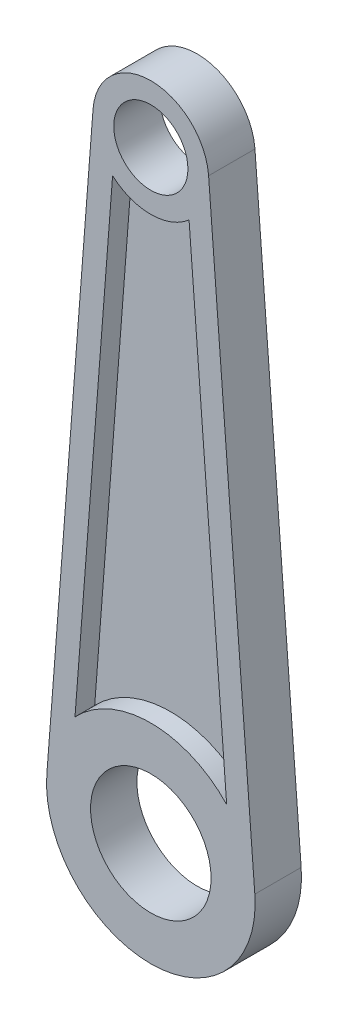
from build123d import *

# Parameters (mm, degrees)
ROD_PROFILE_SKETCH_R   = 8
ROD_PROFILE_SKETCH_R_2 = 13
ROD_BODY_10MM_DEPTH    = 5
WEB_RECESS_1_5MM_DEPTH = 0.75


with BuildPart() as part:
    # Rod Profile Sketch → Rod Body 10mm (new, symmetric)
    with BuildSketch(Plane.XY):
        with BuildLine():
            Line((-12.462962882, 65.961538462), (-22.433333187, -63.269230769))
            ThreePointArc((-22.433333187, -63.269230769), (0, -87.5), (22.433333187, -63.269230769))
            Line((22.433333187, -63.269230769), (12.462962882, 65.961538462))
            ThreePointArc((12.462962882, 65.961538462), (0, 77.5), (-12.462962882, 65.961538462))
        make_face()
        with Locations((0, 65)):
            Circle(ROD_PROFILE_SKETCH_R, mode=Mode.SUBTRACT)
        with Locations((0, -65)):
            Circle(ROD_PROFILE_SKETCH_R_2, mode=Mode.SUBTRACT)
        with BuildLine():
            Line((-8.247008498, 55.606552772), (-16.360291448, -49.553613246))
            ThreePointArc((-16.360291448, -49.553613246), (0, -42.5), (16.360291448, -49.553613246))
            Line((16.360291448, -49.553613246), (8.247008498, 55.606552772))
            ThreePointArc((8.247008498, 55.606552772), (0, 52.5), (-8.247008498, 55.606552772))
        make_face(mode=Mode.SUBTRACT)
    extrude(amount=ROD_BODY_10MM_DEPTH, both=True)

    # Sketch1_3 → Web Recess 1.5mm (add, symmetric)
    with BuildSketch(Plane.XY):
        with BuildLine():
            ThreePointArc((16.360291448, -49.553613246), (0, -42.5), (-16.360291448, -49.553613246))
            Line((-16.360291448, -49.553613246), (-8.247008498, 55.606552772))
            ThreePointArc((-8.247008498, 55.606552772), (0, 52.5), (8.247008498, 55.606552772))
            Line((8.247008498, 55.606552772), (16.360291448, -49.553613246))
        make_face()
    extrude(amount=WEB_RECESS_1_5MM_DEPTH, both=True)


solid = part.part
